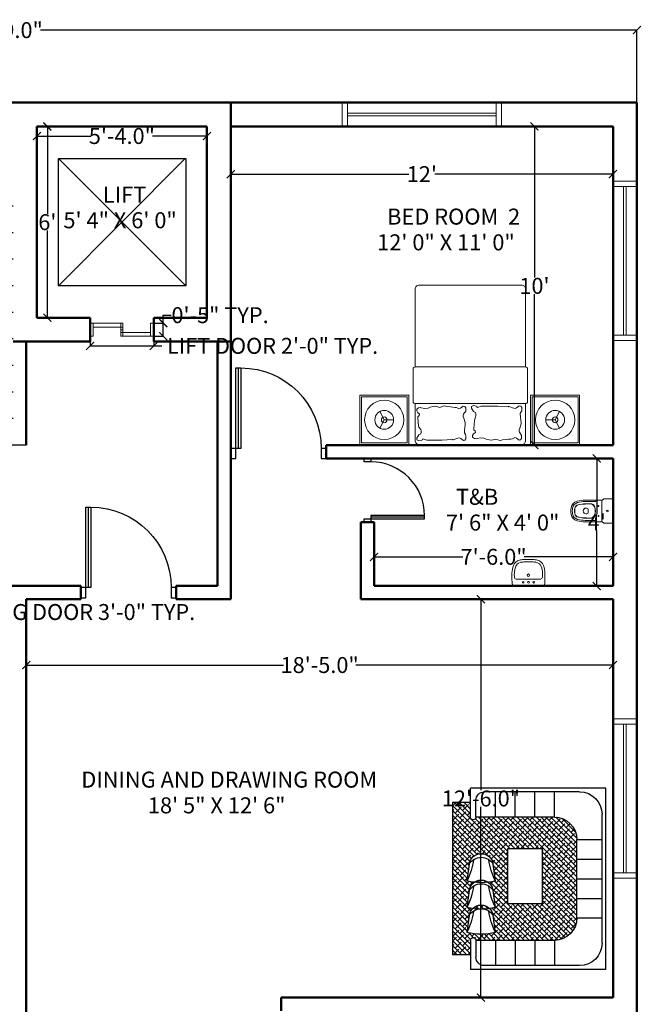
# Model space of a CAD drawing. Units: inches. Extents: x 147 to 1638, y 107 to 941.
# Tile 11 of 17: x 469 to 704, y 570 to 941. Entities that reach past the tile are written whole.
import ezdxf

# ---------------------------------------------------------------- set-up
doc = ezdxf.new("R2010")
doc.units = ezdxf.units.IN
doc.header["$MEASUREMENT"] = 0
for name, color, linetype, lineweight in [('A-ANNO-DIMS', 2, 'Continuous', 15), ('A-AREA-IDEN', 7, 'Continuous', 18), ('A-Door', 150, 'Continuous', 25), ('A-EQPM-ELEV', 7, 'Continuous', 25), ('A-FLOR-FIXT', 9, 'Continuous', 18), ('A-FLOR-STRS', 7, 'Continuous', 25), ('furniture', 50, 'Continuous', 18), ('HAT', 9, 'Continuous', 0), ('lift door', 200, 'Continuous', 20), ('walls', 7, 'Continuous', 50), ('windows', 3, 'Continuous', 20)]:
    doc.layers.add(name, color=color, linetype=linetype, lineweight=lineweight)
for name, color, linetype in [('A-Glaz', 92, 'Continuous'), ('FUR', 42, 'Continuous'), ('NT', 1, 'Continuous'), ('Win', 152, 'Continuous')]:
    doc.layers.add(name, color=color, linetype=linetype)
doc.styles.get("Standard").update_dxf_attribs({"font": 'arial.ttf'})
doc.dimstyles.get("Standard").update_dxf_attribs({"dimtxt": 6, "dimasz": 3, "dimexe": 0.18, "dimexo": 0.0625, "dimgap": 0.09, "dimtad": 0, "dimtih": 1, "dimtoh": 1, "dimdec": 1, "dimzin": 0, "dimdsep": 46, "dimlunit": 3, "dimtxsty": 'Standard', "dimblk": 'ARCHTICK', "dimcen": 0.09, "dimadec": 0, "dimazin": 0, "dimtfac": 1, "dimtdec": 1, "dimtofl": 0, "dimtmove": 0, "dimatfit": 3, "dimfxl": 1, "dimtolj": 1, "dimtzin": 0, "dimarcsym": 0})

# ---------------------------------------------------------------- blocks, each defined once
blk = doc.blocks.new('A$C087A3AA9')
at = {"layer": 'A-Door'}
for points in [[(852.6, 94.7), (852.6, 852.6), (805.3, 852.6), (805.3, 94.7)], [(47.4, 94.7), (47.4, 0), (0, 0), (0, 94.7)], [(900, 94.7), (900, 0), (852.6, 0), (852.6, 94.7)]]:
    blk.add_lwpolyline(points, close=True, dxfattribs=at)
at = {"layer": 'A-Glaz'}
blk.add_line((828.9, 852.6), (828.9, 94.7), dxfattribs=at)
at = {"layer": 'NT'}
blk.add_arc((805.3, 94.7), 757.9, 90, 180, dxfattribs=at)
blk = doc.blocks.new('_ArchTick')
at = {"color": 0, "linetype": 'ByBlock', "const_width": 0.15}
blk.add_lwpolyline([(-0.5, -0.5), (0.5, 0.5)], dxfattribs=at)
blk = doc.blocks.new('*D5')
at = {"layer": 'A-ANNO-DIMS', "color": 0, "lineweight": -2, "transparency": 16777216}
for p, q in [((666.77, 900.72), (663.17, 900.72)), ((663.35, 900.72), (663.35, 843.87)), ((663.35, 780.72), (663.35, 837.56)), ((666.77, 780.72), (663.17, 780.72))]:
    blk.add_line(p, q, dxfattribs=at)
at = {"layer": 'Defpoints', "color": 0, "lineweight": -2, "transparency": 16777216}
for p in [(666.83, 900.72), (663.35, 780.72), (666.83, 780.72)]:
    blk.add_point(p, dxfattribs=at)
at = {"layer": 'A-ANNO-DIMS', "color": 0, "lineweight": -2, "transparency": 16777216, "xscale": 3, "yscale": 3, "zscale": 3}
for p, rotation in [((663.35, 900.72), 90), ((663.35, 780.72), 270)]:
    blk.add_blockref('_ArchTick', p, dxfattribs=dict(at, rotation=rotation))
at = {"layer": 'A-ANNO-DIMS', "color": 0, "transparency": 16777216, "insert": (663.35, 840.72), "char_height": 6, "attachment_point": 5}
blk.add_mtext("\\A1;10'", dxfattribs=at)
blk = doc.blocks.new('*D6')
at = {"layer": 'A-ANNO-DIMS', "color": 0, "lineweight": -2, "transparency": 16777216}
for p, q in [((548.94, 882.79), (616.05, 882.79)), ((548.94, 882.73), (548.94, 882.61)), ((692.94, 882.79), (625.84, 882.79)), ((692.94, 882.85), (692.94, 882.97))]:
    blk.add_line(p, q, dxfattribs=at)
at = {"layer": 'Defpoints', "color": 0, "lineweight": -2, "transparency": 16777216}
for p in [(548.94, 882.79), (692.94, 882.79), (692.94, 882.79)]:
    blk.add_point(p, dxfattribs=at)
at = {"layer": 'A-ANNO-DIMS', "color": 0, "lineweight": -2, "transparency": 16777216, "xscale": 3, "yscale": 3, "zscale": 3, "rotation": 180}
blk.add_blockref('_ArchTick', (548.94, 882.79), dxfattribs=at)
at = {"layer": 'A-ANNO-DIMS', "color": 0, "lineweight": -2, "transparency": 16777216, "xscale": 3, "yscale": 3, "zscale": 3}
blk.add_blockref('_ArchTick', (692.94, 882.79), dxfattribs=at)
at = {"layer": 'A-ANNO-DIMS', "color": 0, "transparency": 16777216, "insert": (620.94, 882.79), "char_height": 6, "attachment_point": 5}
blk.add_mtext("\\A1;12'", dxfattribs=at)
blk = doc.blocks.new('*D10')
at = {"layer": 'A-ANNO-DIMS', "color": 0, "lineweight": -2, "transparency": 16777216}
for p, q in [((687.62, 775.72), (686.65, 775.72)), ((686.83, 775.72), (686.83, 754.81)), ((686.83, 727.72), (686.83, 748.63)), ((687.62, 727.72), (686.65, 727.72))]:
    blk.add_line(p, q, dxfattribs=at)
at = {"layer": 'Defpoints', "color": 0, "lineweight": -2, "transparency": 16777216}
for p in [(687.68, 775.72), (686.83, 727.72), (687.68, 727.72)]:
    blk.add_point(p, dxfattribs=at)
at = {"layer": 'A-ANNO-DIMS', "color": 0, "lineweight": -2, "transparency": 16777216, "xscale": 3, "yscale": 3, "zscale": 3}
for p, rotation in [((686.83, 775.72), 90), ((686.83, 727.72), 270)]:
    blk.add_blockref('_ArchTick', p, dxfattribs=dict(at, rotation=rotation))
at = {"layer": 'A-ANNO-DIMS', "color": 0, "transparency": 16777216, "insert": (686.83, 751.72), "char_height": 6, "attachment_point": 5}
blk.add_mtext("\\A1;4'", dxfattribs=at)
blk = doc.blocks.new('*D11')
at = {"layer": 'A-ANNO-DIMS', "color": 0, "lineweight": -2, "transparency": 16777216}
for p, q in [((602.94, 736.98), (602.94, 738.87)), ((602.94, 738.69), (636.41, 738.69)), ((692.94, 738.69), (659.48, 738.69)), ((692.94, 736.98), (692.94, 738.87))]:
    blk.add_line(p, q, dxfattribs=at)
at = {"layer": 'Defpoints', "color": 0, "lineweight": -2, "transparency": 16777216}
for p in [(692.94, 738.69), (602.94, 736.92), (692.94, 736.92)]:
    blk.add_point(p, dxfattribs=at)
at = {"layer": 'A-ANNO-DIMS', "color": 0, "lineweight": -2, "transparency": 16777216, "xscale": 3, "yscale": 3, "zscale": 3, "rotation": 180}
blk.add_blockref('_ArchTick', (602.94, 738.69), dxfattribs=at)
at = {"layer": 'A-ANNO-DIMS', "color": 0, "lineweight": -2, "transparency": 16777216, "xscale": 3, "yscale": 3, "zscale": 3}
blk.add_blockref('_ArchTick', (692.94, 738.69), dxfattribs=at)
at = {"layer": 'A-ANNO-DIMS', "color": 0, "transparency": 16777216, "insert": (647.94, 738.69), "char_height": 6, "attachment_point": 5}
blk.add_mtext('\\A1;7\'-6.0"', dxfattribs=at)
blk = doc.blocks.new('*D26')
at = {"layer": 'A-ANNO-DIMS', "color": 0, "lineweight": -2, "transparency": 16777216}
for p, q in [((650.57, 722.72), (643.01, 722.72)), ((643.19, 722.72), (643.19, 650.87)), ((643.19, 572.72), (643.19, 644.56)), ((650.57, 572.72), (643.01, 572.72))]:
    blk.add_line(p, q, dxfattribs=at)
at = {"layer": 'Defpoints', "color": 0, "lineweight": -2, "transparency": 16777216}
for p in [(650.64, 722.72), (643.19, 572.72), (650.64, 572.72)]:
    blk.add_point(p, dxfattribs=at)
at = {"layer": 'A-ANNO-DIMS', "color": 0, "lineweight": -2, "transparency": 16777216, "xscale": 3, "yscale": 3, "zscale": 3}
for p, rotation in [((643.19, 722.72), 90), ((643.19, 572.72), 270)]:
    blk.add_blockref('_ArchTick', p, dxfattribs=dict(at, rotation=rotation))
at = {"layer": 'A-ANNO-DIMS', "color": 0, "transparency": 16777216, "insert": (643.19, 647.72), "char_height": 6, "attachment_point": 5}
blk.add_mtext('\\A1;12\'-6.0"', dxfattribs=at)
blk = doc.blocks.new('*D27')
at = {"layer": 'A-ANNO-DIMS', "color": 0, "lineweight": -2, "transparency": 16777216}
for p, q in [((471.94, 695.66), (471.94, 698.14)), ((471.94, 697.96), (568.84, 697.96)), ((692.94, 697.96), (596.05, 697.96)), ((692.94, 695.66), (692.94, 698.14))]:
    blk.add_line(p, q, dxfattribs=at)
at = {"layer": 'Defpoints', "color": 0, "lineweight": -2, "transparency": 16777216}
for p in [(692.94, 697.96), (471.94, 695.6), (692.94, 695.6)]:
    blk.add_point(p, dxfattribs=at)
at = {"layer": 'A-ANNO-DIMS', "color": 0, "lineweight": -2, "transparency": 16777216, "xscale": 3, "yscale": 3, "zscale": 3, "rotation": 180}
blk.add_blockref('_ArchTick', (471.94, 697.96), dxfattribs=at)
at = {"layer": 'A-ANNO-DIMS', "color": 0, "lineweight": -2, "transparency": 16777216, "xscale": 3, "yscale": 3, "zscale": 3}
blk.add_blockref('_ArchTick', (692.94, 697.96), dxfattribs=at)
at = {"layer": 'A-ANNO-DIMS', "color": 0, "transparency": 16777216, "insert": (582.44, 697.96), "char_height": 6, "attachment_point": 5}
blk.add_mtext('\\A1;18\'-5.0"', dxfattribs=at)
blk = doc.blocks.new('*D32')
at = {"layer": 'A-ANNO-DIMS', "color": 0, "lineweight": -2, "transparency": 16777216}
for p, q in [((475.94, 897.2), (475.94, 897.32)), ((539.94, 897.2), (539.94, 897.32)), ((475.94, 897.14), (496.38, 897.14)), ((539.94, 897.14), (519.5, 897.14))]:
    blk.add_line(p, q, dxfattribs=at)
at = {"layer": 'Defpoints', "color": 0, "lineweight": -2, "transparency": 16777216}
for p in [(475.94, 897.14), (539.94, 897.14), (539.94, 897.14)]:
    blk.add_point(p, dxfattribs=at)
at = {"layer": 'A-ANNO-DIMS', "color": 0, "lineweight": -2, "transparency": 16777216, "xscale": 3, "yscale": 3, "zscale": 3, "rotation": 180}
blk.add_blockref('_ArchTick', (475.94, 897.14), dxfattribs=at)
at = {"layer": 'A-ANNO-DIMS', "color": 0, "lineweight": -2, "transparency": 16777216, "xscale": 3, "yscale": 3, "zscale": 3}
blk.add_blockref('_ArchTick', (539.94, 897.14), dxfattribs=at)
at = {"layer": 'A-ANNO-DIMS', "color": 0, "transparency": 16777216, "insert": (507.94, 897.14), "char_height": 6, "attachment_point": 5}
blk.add_mtext('\\A1;5\'-4.0"', dxfattribs=at)
blk = doc.blocks.new('*D33')
at = {"layer": 'A-ANNO-DIMS', "color": 0, "lineweight": -2, "transparency": 16777216}
for p, q in [((479.9, 900.72), (479.68, 900.72)), ((479.86, 900.72), (479.86, 867.87)), ((479.86, 828.72), (479.86, 861.56)), ((479.9, 828.72), (479.68, 828.72))]:
    blk.add_line(p, q, dxfattribs=at)
at = {"layer": 'Defpoints', "color": 0, "lineweight": -2, "transparency": 16777216}
for p in [(479.96, 900.72), (479.86, 828.72), (479.96, 828.72)]:
    blk.add_point(p, dxfattribs=at)
at = {"layer": 'A-ANNO-DIMS', "color": 0, "lineweight": -2, "transparency": 16777216, "xscale": 3, "yscale": 3, "zscale": 3}
for p, rotation in [((479.86, 900.72), 90), ((479.86, 828.72), 270)]:
    blk.add_blockref('_ArchTick', p, dxfattribs=dict(at, rotation=rotation))
at = {"layer": 'A-ANNO-DIMS', "color": 0, "transparency": 16777216, "insert": (479.86, 864.72), "char_height": 6, "attachment_point": 5}
blk.add_mtext("\\A1;6'", dxfattribs=at)
blk = doc.blocks.new('*D69')
at = {"layer": 'A-ANNO-DIMS', "color": 0, "lineweight": -2, "transparency": 16777216}
for p, q in [((224.94, 909.78), (224.94, 937.18)), ((224.94, 937), (449.56, 937)), ((701.94, 937), (477.33, 937)), ((701.94, 909.78), (701.94, 937.18))]:
    blk.add_line(p, q, dxfattribs=at)
at = {"layer": 'Defpoints', "color": 0, "lineweight": -2, "transparency": 16777216}
for p in [(701.94, 937), (224.94, 909.72), (701.94, 909.72)]:
    blk.add_point(p, dxfattribs=at)
at = {"layer": 'A-ANNO-DIMS', "color": 0, "lineweight": -2, "transparency": 16777216, "xscale": 3, "yscale": 3, "zscale": 3, "rotation": 180}
blk.add_blockref('_ArchTick', (224.94, 937), dxfattribs=at)
at = {"layer": 'A-ANNO-DIMS', "color": 0, "lineweight": -2, "transparency": 16777216, "xscale": 3, "yscale": 3, "zscale": 3}
blk.add_blockref('_ArchTick', (701.94, 937), dxfattribs=at)
at = {"layer": 'A-ANNO-DIMS', "color": 0, "transparency": 16777216, "insert": (463.44, 937), "char_height": 6, "attachment_point": 5}
blk.add_mtext('\\A1;39\'-9.0"', dxfattribs=at)
blk = doc.blocks.new('MAT-P14')
for p, q in [((-1.337, 1.348), (-1.337, 1.948)), ((-1.337, 1.948), (-0.737, 1.948)), ((-1.317, 1.928), (-0.757, 1.928)), ((-1.317, 1.368), (-1.317, 1.928)), ((-0.757, 1.368), (-0.757, 1.928)), ((-0.737, 1.348), (-0.737, 1.948)), ((0.625, 1.95), (-0.625, 1.95)), ((0.753, 1.348), (0.753, 1.948)), ((1.353, 1.948), (0.753, 1.948)), ((1.333, 1.928), (0.773, 1.928)), ((0.773, 1.368), (0.773, 1.928)), ((1.333, 1.368), (1.333, 1.928)), ((1.353, 1.348), (1.353, 1.948)), ((-1.037, 1.648), (-1.091, 1.749)), ((1.053, 1.648), (1.108, 1.749)), ((-1.037, 1.648), (-1.091, 1.547)), ((-1.037, 1.648), (-0.922, 1.648)), ((1.053, 1.648), (0.938, 1.648)), ((1.053, 1.648), (1.108, 1.547)), ((-1.337, 1.348), (-0.737, 1.348)), ((-1.317, 1.368), (-0.757, 1.368)), ((1.353, 1.348), (0.753, 1.348)), ((1.333, 1.368), (0.773, 1.368))]:
    blk.add_line(p, q)
for points in [[(-0.675, 1.45), (-0.675, 1.9, -0.414214), (-0.625, 1.95), (0.625, 1.95, -0.414214), (0.675, 1.9), (0.675, 1.45)], [(-0.675, 1, -0.414214), (-0.7, 1.025), (-0.7, 1.425, -0.414214), (-0.675, 1.45), (0.675, 1.45, -0.414214), (0.7, 1.425), (0.7, 1.025, -0.414214), (0.675, 1)], [(-0.625, 0, -0.414214), (-0.675, 0.05), (-0.675, 1), (0.675, 1), (0.675, 0.05, -0.414214), (0.625, 0)]]:
    blk.add_lwpolyline(points, format="xyb", close=True)
blk.add_lwpolyline([(-0.542, 1.95), (-0.542, 1.967), (0.558, 1.967), (0.558, 1.95)], close=True)
for points in [[(-0.614, 1.818), (-0.626, 1.838), (-0.626, 1.877), (-0.614, 1.891), (-0.596, 1.896), (-0.579, 1.886), (-0.563, 1.872), (-0.545, 1.863), (-0.516, 1.879), (-0.497, 1.882), (-0.465, 1.884), (-0.439, 1.887), (-0.395, 1.892), (-0.363, 1.9), (-0.309, 1.882), (-0.262, 1.897), (-0.23, 1.892), (-0.192, 1.884), (-0.166, 1.873), (-0.128, 1.868), (-0.082, 1.875), (-0.076, 1.88), (-0.052, 1.875), (-0.028, 1.861), (-0.028, 1.841), (-0.04, 1.817), (-0.064, 1.802), (-0.06, 1.781), (-0.043, 1.768), (-0.046, 1.697), (-0.05, 1.662), (-0.056, 1.64), (-0.062, 1.612), (-0.068, 1.596), (-0.068, 1.579), (-0.063, 1.56), (-0.039, 1.545), (-0.015, 1.505), (-0.015, 1.486), (-0.038, 1.471), (-0.075, 1.482), (-0.081, 1.487), (-0.087, 1.497), (-0.134, 1.481), (-0.304, 1.482), (-0.318, 1.482), (-0.335, 1.479), (-0.464, 1.488), (-0.467, 1.486), (-0.473, 1.486), (-0.517, 1.503), (-0.53, 1.505), (-0.548, 1.51), (-0.566, 1.501), (-0.581, 1.487), (-0.599, 1.477), (-0.617, 1.482), (-0.629, 1.497), (-0.629, 1.536), (-0.623, 1.55), (-0.611, 1.57), (-0.614, 1.614), (-0.615, 1.627), (-0.618, 1.644), (-0.619, 1.66), (-0.62, 1.675), (-0.62, 1.695), (-0.618, 1.707), (-0.614, 1.723), (-0.608, 1.739), (-0.604, 1.75), (-0.598, 1.771), (-0.596, 1.785), (-0.6, 1.798), (-0.614, 1.819)], [(0.069, 1.559), (0.057, 1.54), (0.057, 1.501), (0.069, 1.486), (0.087, 1.481), (0.105, 1.491), (0.121, 1.505), (0.139, 1.514), (0.168, 1.498), (0.187, 1.496), (0.219, 1.493), (0.244, 1.49), (0.289, 1.485), (0.321, 1.477), (0.374, 1.495), (0.422, 1.48), (0.454, 1.486), (0.492, 1.493), (0.517, 1.504), (0.555, 1.509), (0.602, 1.502), (0.608, 1.497), (0.632, 1.502), (0.656, 1.517), (0.656, 1.536), (0.644, 1.561), (0.62, 1.575), (0.624, 1.596), (0.641, 1.609), (0.637, 1.68), (0.633, 1.715), (0.628, 1.738), (0.606, 1.765), (0.6, 1.781), (0.6, 1.798), (0.605, 1.817), (0.629, 1.832), (0.654, 1.872), (0.654, 1.892), (0.63, 1.906), (0.593, 1.895), (0.587, 1.891), (0.581, 1.881), (0.534, 1.896), (0.379, 1.896), (0.366, 1.896), (0.348, 1.898), (0.22, 1.89), (0.216, 1.891), (0.21, 1.891), (0.167, 1.875), (0.154, 1.872), (0.136, 1.867), (0.118, 1.876), (0.102, 1.89), (0.085, 1.9), (0.067, 1.895), (0.055, 1.881), (0.055, 1.842), (0.061, 1.827), (0.073, 1.807), (0.07, 1.764), (0.069, 1.75), (0.066, 1.733), (0.065, 1.718), (0.063, 1.703), (0.063, 1.682), (0.066, 1.67), (0.07, 1.655), (0.075, 1.638), (0.079, 1.627), (0.086, 1.607), (0.087, 1.592), (0.083, 1.579), (0.07, 1.559)]]:
    blk.add_lwpolyline(points)
for centre, radius in [((-1.037, 1.648), 0.24), ((1.053, 1.648), 0.24), ((-1.037, 1.648), 0.115), ((1.053, 1.648), 0.115), ((-1.037, 1.648), 0.035), ((1.053, 1.648), 0.035)]:
    blk.add_circle(centre, radius)
blk = doc.blocks.new('2SAINDA')
at = {"color": 0, "linetype": 'ByBlock'}
for p, q in [((0, 0.188), (0, -0.188)), ((0.018, 0.2), (0.141, 0.2)), ((0.157, 0.192), (0.162, 0.188)), ((0.18, -0.164), (0.18, 0.164)), ((0.279, 0.159), (0.261, 0.176)), ((0.437, 0.047), (0.424, 0.047)), ((0.279, -0.159), (0.261, -0.176)), ((0.437, -0.047), (0.424, -0.047)), ((0.018, -0.2), (0.141, -0.2)), ((0.157, -0.192), (0.162, -0.188))]:
    blk.add_line(p, q, dxfattribs=at)
for centre, radius in [((0.09, 0), 0.0135), ((0.09, 0), 0.0135), ((0.236, 0.08), 0.0075), ((0.236, -0.08), 0.0075)]:
    blk.add_circle(centre, radius, dxfattribs=at)
for centre, radius, start, end in [((0.018, 0.18), 0.02, 90, 155.6901), ((0.141, 0.181), 0.019, 34.9372, 90), ((0.155, 0.164), 0.025, 23.3776, 73.7848), ((0.383, -5.322), 5.5, 89.2905, 92.1362), ((0.155, 0.164), 0.025, 360, 23.3776), ((0.444, -0.373), 0.55, 75.4605, 89.2905), ((0.293, 0.173), 0.02, 225, 270.9364), ((0.485, 0), 0.2, 160.016, 199.984), ((0.485, 0), 0.196, 160.016, 199.984), ((0.383, -5.322), 5.476, 89.2905, 90.9364), ((0.368, 0.043), 0.075, 90.1648, 160.016), ((0.368, 0.043), 0.071, 90.1648, 160.016), ((0.383, -5.322), 5.44, 89.2905, 90.1648), ((0.383, -5.322), 5.436, 89.2905, 90.1648), ((0.582, 0), 0.18, 170.2849, 189.7151), ((0.424, 0.027), 0.02, 90, 170.2849), ((0.437, 0), 0.047, 0, 90), ((0.437, 0), 0.047, 270, 0), ((0.444, -0.373), 0.49, 75.4605, 89.2905), ((0.444, -0.373), 0.486, 75.4605, 89.2905), ((0.444, -0.373), 0.526, 75.4605, 89.2905), ((0.549, 0.03), 0.07, 8.8162, 75.4605), ((0.549, 0.03), 0.074, 8.8162, 75.4605), ((0.549, 0.03), 0.11, 8.8162, 75.4605), ((0.549, 0.03), 0.134, 8.8162, 75.4605), ((0.355, 0), 0.266, 351.1838, 8.8162), ((0.355, 0), 0.27, 351.1838, 8.8162), ((0.355, 0), 0.306, 351.1838, 8.8162), ((0.355, 0), 0.33, 351.1838, 8.8162), ((0.293, -0.173), 0.02, 89.0636, 135), ((0.383, 5.322), 5.476, 269.0636, 270.7095), ((0.368, -0.043), 0.075, 199.984, 269.8352), ((0.368, -0.043), 0.071, 199.984, 269.8352), ((0.383, 5.322), 5.436, 269.8352, 270.7095), ((0.383, 5.322), 5.44, 269.8352, 270.7095), ((0.424, -0.027), 0.02, 189.7151, 270), ((0.444, 0.373), 0.486, 270.7095, 284.5395), ((0.444, 0.373), 0.49, 270.7095, 284.5395), ((0.444, 0.373), 0.526, 270.7095, 284.5395), ((0.444, 0.373), 0.55, 270.7095, 284.5395), ((0.549, -0.03), 0.07, 284.5395, 351.1838), ((0.549, -0.03), 0.074, 284.5395, 351.1838), ((0.549, -0.03), 0.11, 284.5395, 351.1838), ((0.549, -0.03), 0.134, 284.5395, 351.1838), ((0.018, -0.18), 0.02, 204.3099, 270), ((0.141, -0.181), 0.019, 270, 325.0628), ((0.155, -0.164), 0.025, 286.2152, 336.6224), ((0.155, -0.164), 0.025, 336.6224, 0), ((0.383, 5.322), 5.5, 267.8638, 270.7095)]:
    blk.add_arc(centre, radius, start, end, dxfattribs=at)
blk = doc.blocks.new('2SALADA2')
at = {"color": 0}
for p, q in [((-0.296, 0), (0.296, 0)), ((0.207, -0.13), (-0.207, -0.13))]:
    blk.add_line(p, q, dxfattribs=at)
for centre, radius in [((-0.1, -0.07), 0.015), ((0, -0.205), 0.023), ((0, -0.07), 0.0175), ((0.1, -0.07), 0.015)]:
    blk.add_circle(centre, radius, dxfattribs=at)
for centre, radius, start, end in [((-0.296, -0.01), 0.01, 90, 173.6262), ((0.296, -0.01), 0.01, 6.3738, 90), ((1.185, -0.175), 1.5, 173.6262, 182.693), ((1.186, -0.221), 1.454, 178.0234, 180.898), ((-0.227, -0.171), 0.04, 95.5937, 179.6995), ((-0.207, -0.38), 0.25, 90, 95.5937), ((0.207, -0.38), 0.25, 84.4063, 90), ((0.227, -0.171), 0.04, 0.3005, 84.4063), ((-1.186, -0.221), 1.454, 359.102, 1.9766), ((-1.185, -0.175), 1.5, 357.307, 6.3738), ((0.186, -0.222), 0.5, 182.693, 199.3406), ((0.186, -0.222), 0.454, 182.693, 199.3406), ((-0.135, -0.335), 0.114, 199.3406, 257.4429), ((0.135, -0.335), 0.114, 282.5571, 340.6594), ((-0.186, -0.222), 0.454, 340.6594, 357.307), ((-0.186, -0.222), 0.5, 340.6594, 357.307), ((-0.135, -0.335), 0.16, 199.3406, 257.4429), ((-0.061, -0.003), 0.5, 257.4429, 266.4982), ((-0.061, -0.003), 0.454, 257.4429, 266.4982), ((0, 0.995), 1.5, 266.4982, 273.5018), ((0, 0.995), 1.454, 266.4982, 273.5018), ((0.061, -0.003), 0.454, 273.5018, 282.5571), ((0.061, -0.003), 0.5, 273.5018, 282.5571), ((0.135, -0.335), 0.16, 282.5571, 340.6594)]:
    blk.add_arc(centre, radius, start, end, dxfattribs=at)
blk = doc.blocks.new('CHAIR1')
for p, q in [((-393, -750), (-329, -287)), ((329, -286), (394, -750))]:
    blk.add_line(p, q)
for centre, radius, start, end in [((0, -332), 332, 7.9072, 172.1612), ((-1856, 27), 1657, 332.0394, 353.4161), ((0, -483), 383, 30.9021, 149.1663), ((1857, 27), 1657, 186.5839, 207.9606), ((0, 770), 1570, 255.502, 284.498)]:
    blk.add_arc(centre, radius, start, end)
blk = doc.blocks.new('A$C1CFC4E3A')
at = {"layer": 'HAT'}
h = blk.add_hatch(dxfattribs=at)
h.set_pattern_fill('ANSI38,_O', color=256, scale=0.664121)
h.set_pattern_definition([(45, (6.13299, -18.48134), (-0.05870057, 0.05870057), []), (135, (6.13299, -18.48134), (-0.1761017, 0.05870057), [0.2075378, -0.1245227])])
h.paths.add_polyline_path([(0, 3.705), (-0.438, 3.705), (-0.438, 3.353, -1), (-0.573, 3.353), (-2.482, 3.353, 0.414214), (-3.028, 2.807), (-3.028, 0.898, 0.414214), (-2.482, 0.352), (-0.573, 0.352, -1), (-0.438, 0.352), (-0.438, 0), (0, 0)])
h.paths.add_polyline_path([(-1.342, 1.248), (-2.191, 1.248), (-2.191, 2.58), (-1.342, 2.58)], flags=16)
h.paths.add_polyline_path([(-0.409, 1.566), (-0.352, 1.156, -0.127199), (-1.048, 1.156), (-0.992, 1.566, -0.871235)], flags=16)
h.paths.add_polyline_path([(-0.409, 0.959), (-0.352, 0.548, -0.127199), (-1.048, 0.548), (-0.992, 0.958, -0.871235)], flags=16)
h.paths.add_polyline_path([(-0.992, 2.209, -0.871235), (-0.409, 2.21), (-0.352, 1.799, -0.127199), (-1.048, 1.799)], flags=16)
at = {"layer": 'FUR'}
for p, q in [((-3.732, 4.057), (-0.438, 4.057)), ((-3.732, -0.352), (-3.732, 4.057)), ((-3.096, 3.967), (-0.777, 3.967)), ((-2.482, 3.353), (-2.482, 3.967)), ((-2.005, 3.353), (-2.005, 3.967)), ((-1.528, 3.353), (-1.528, 3.967)), ((-1.05, 3.353), (-1.05, 3.967)), ((-0.438, 3.353), (-0.438, 4.057)), ((-0.573, 3.353), (-0.573, 3.762)), ((-3.642, 0.284), (-3.642, 3.421)), ((-2.482, 3.353), (-0.573, 3.353)), ((-3.028, 2.807), (-3.642, 2.807)), ((-3.028, 2.33), (-3.642, 2.33)), ((-3.028, 1.852), (-3.642, 1.852)), ((-3.028, 1.375), (-3.642, 1.375)), ((-3.028, 0.898), (-3.642, 0.898)), ((-2.482, 0.352), (-0.573, 0.352)), ((-2.482, 0.352), (-2.482, -0.262)), ((-2.005, 0.352), (-2.005, -0.262)), ((-1.528, 0.352), (-1.528, -0.262)), ((-1.05, 0.352), (-1.05, -0.262)), ((-0.573, 0.352), (-0.573, -0.057)), ((-0.438, 0.352), (-0.438, -0.352)), ((-3.732, -0.352), (-0.438, -0.352)), ((-3.096, -0.262), (-0.777, -0.262))]:
    blk.add_line(p, q, dxfattribs=at)
for centre, radius, start, end in [((-3.096, 3.421), 0.546, 90, 180), ((-0.777, 3.762), 0.205, 0, 90), ((-2.482, 2.807), 0.546, 90, 180), ((-0.505, 3.353), 0.0675, 180, 0), ((-2.482, 0.898), 0.546, 180, 270), ((-3.096, 0.284), 0.546, 180, 270), ((-0.505, 0.352), 0.0675, 0, 180), ((-0.777, -0.057), 0.205, 270, 0)]:
    blk.add_arc(centre, radius, start, end, dxfattribs=at)
at = {"layer": 'Win'}
for p, q in [((-0.438, 3.705), (0, 3.705)), ((0, 3.705), (0, 0)), ((-3.028, 0.898), (-3.028, 2.807)), ((-0.438, 0), (0, 0))]:
    blk.add_line(p, q, dxfattribs=at)
blk.add_lwpolyline([(-2.191, 2.58), (-1.342, 2.58), (-1.342, 1.248), (-2.191, 1.248)], close=True, dxfattribs=at)
at = {"layer": 'FUR', "xscale": 0.0008854948152227, "yscale": 0.0008854948152227, "zscale": 0.0008854948152227}
for p in [(-0.7, 2.463), (-0.7, 1.82), (-0.7, 1.212)]:
    blk.add_blockref('CHAIR1', p, dxfattribs=at)
blk = doc.blocks.new('WIN-60IN')
for p, q in [((60, 9), (0, 9)), ((0, 9), (0, 0)), ((2, 9), (2, 0)), ((58, 0), (58, 9)), ((60, 0), (60, 9)), ((2, 5), (58, 5)), ((2, 4), (58, 4)), ((0, 0), (60, 0))]:
    blk.add_line(p, q)
blk = doc.blocks.new('LIFT-CAR')
for p, q in [((48, 0), (0, 48)), ((47.77, 48), (0, 0))]:
    blk.add_line(p, q)
blk.add_lwpolyline([(0, 48), (48, 48), (48, 0), (0, 0)], close=True)
blk = doc.blocks.new('LIFT-DOOR-CENTER-OPEN')
for p, q in [((1.24, 4.95), (12.38, 4.95)), ((11.62, 2.48), (11.62, 4.95)), ((12.38, 4.95), (12.38, 2.48)), ((1.24, 3.49), (12.38, 3.49)), ((11.62, 0), (11.62, 2.48)), ((11.62, 2.48), (12.38, 2.48)), ((12.38, 2.48), (11.62, 2.48)), ((22.76, 1.47), (11.62, 1.47)), ((12.38, 2.48), (12.38, 0)), ((22.76, 0), (11.62, 0))]:
    blk.add_line(p, q)
for points in [[(1.24, 0), (0, 0), (0, 4.95), (1.24, 4.95)], [(22.76, 4.95), (24, 4.95), (24, 0), (22.76, 0)]]:
    blk.add_lwpolyline(points, close=True)
blk = doc.blocks.new('STAIR-RETURN-FLIGHTS')
for p, q in [((0, 90), (36, 90)), ((36, 0), (36, 90)), ((36, 90), (48, 90)), ((84, 90), (48, 90)), ((48, 90), (48, 0)), ((0, 80), (36, 80)), ((84, 80), (48, 80)), ((0, 70), (36, 70)), ((84, 70), (48, 70)), ((0, 60), (36, 60)), ((84, 60), (48, 60)), ((0, 50), (36, 50)), ((84, 50), (48, 50)), ((0, 40), (36, 40)), ((84, 40), (48, 40)), ((0, 30), (36, 30)), ((84, 30), (48, 30)), ((0, 20), (36, 20)), ((84, 20), (48, 20)), ((0, 10), (36, 10)), ((84, 10), (48, 10)), ((0, 0), (36, 0)), ((48, 0), (36, 0)), ((89, 0), (48, 0))]:
    blk.add_line(p, q)
blk = doc.blocks.new('*D100')
at = {"layer": 'A-ANNO-DIMS', "color": 0, "lineweight": -2, "transparency": 16777216}
for p, q in [((404.44, 723.26), (404.44, 717.74)), ((440.44, 723.26), (440.44, 717.74)), ((404.44, 717.92), (440.44, 717.92)), ((440.44, 717.92), (443.44, 717.92))]:
    blk.add_line(p, q, dxfattribs=at)
at = {"layer": 'Defpoints', "color": 0, "lineweight": -2, "transparency": 16777216}
for p in [(404.44, 723.32), (440.44, 723.32), (440.44, 717.92)]:
    blk.add_point(p, dxfattribs=at)
at = {"layer": 'A-ANNO-DIMS', "color": 0, "lineweight": -2, "transparency": 16777216, "xscale": 3, "yscale": 3, "zscale": 3, "rotation": 180}
blk.add_blockref('_ArchTick', (404.44, 717.92), dxfattribs=at)
at = {"layer": 'A-ANNO-DIMS', "color": 0, "lineweight": -2, "transparency": 16777216, "xscale": 3, "yscale": 3, "zscale": 3}
blk.add_blockref('_ArchTick', (440.44, 717.92), dxfattribs=at)
at = {"layer": 'A-ANNO-DIMS', "color": 0, "transparency": 16777216, "insert": (490.91, 717.92), "char_height": 6, "attachment_point": 5}
blk.add_mtext('\\A1;SWING DOOR 3\'-0" TYP.', dxfattribs=at)
blk = doc.blocks.new('*D130')
at = {"layer": 'A-ANNO-DIMS', "color": 0, "lineweight": -2, "transparency": 16777216}
for p, q in [((495.94, 821.68), (495.94, 817.96)), ((519.94, 821.68), (519.94, 817.96)), ((495.94, 818.14), (519.94, 818.14)), ((519.94, 818.14), (522.94, 818.14))]:
    blk.add_line(p, q, dxfattribs=at)
at = {"layer": 'Defpoints', "color": 0, "lineweight": -2, "transparency": 16777216}
for p in [(495.94, 821.74), (519.94, 821.74), (519.94, 818.14)]:
    blk.add_point(p, dxfattribs=at)
at = {"layer": 'A-ANNO-DIMS', "color": 0, "lineweight": -2, "transparency": 16777216, "xscale": 3, "yscale": 3, "zscale": 3, "rotation": 180}
blk.add_blockref('_ArchTick', (495.94, 818.14), dxfattribs=at)
at = {"layer": 'A-ANNO-DIMS', "color": 0, "lineweight": -2, "transparency": 16777216, "xscale": 3, "yscale": 3, "zscale": 3}
blk.add_blockref('_ArchTick', (519.94, 818.14), dxfattribs=at)
at = {"layer": 'A-ANNO-DIMS', "color": 0, "transparency": 16777216, "insert": (564.7, 818.14), "char_height": 6, "attachment_point": 5}
blk.add_mtext('\\A1;LIFT DOOR 2\'-0" TYP.', dxfattribs=at)
blk = doc.blocks.new('*D131')
at = {"layer": 'A-ANNO-DIMS', "color": 0, "lineweight": -2, "transparency": 16777216}
for p, q in [((523.54, 826.69), (523.54, 829.69)), ((523.54, 829.69), (526.54, 829.69)), ((520.01, 826.69), (523.72, 826.69)), ((523.54, 821.74), (523.54, 826.69)), ((520.01, 821.74), (523.72, 821.74))]:
    blk.add_line(p, q, dxfattribs=at)
at = {"layer": 'Defpoints', "color": 0, "lineweight": -2, "transparency": 16777216}
for p in [(519.94, 826.69), (523.54, 826.69), (519.94, 821.74)]:
    blk.add_point(p, dxfattribs=at)
at = {"layer": 'A-ANNO-DIMS', "color": 0, "lineweight": -2, "transparency": 16777216, "xscale": 3, "yscale": 3, "zscale": 3}
for p, rotation in [((523.54, 826.69), 90), ((523.54, 821.74), 270)]:
    blk.add_blockref('_ArchTick', p, dxfattribs=dict(at, rotation=rotation))
at = {"layer": 'A-ANNO-DIMS', "color": 0, "transparency": 16777216, "insert": (544.92, 829.69), "char_height": 6, "attachment_point": 5}
blk.add_mtext('\\A1;0\'-5" TYP.', dxfattribs=at)

msp = doc.modelspace()

# ---------------------------------------------------------------- linework, layer by layer
at = {"layer": 'walls'}
for p, q in [((224.94, 909.72), (701.94, 909.72)), ((548.94, 909.72), (548.94, 780.72)), ((701.94, 909.72), (701.94, 201.72)), ((475.94, 900.72), (539.94, 900.72)), ((475.94, 900.72), (475.94, 828.72)), ((539.94, 900.72), (539.94, 828.72)), ((548.94, 900.72), (692.94, 900.72)), ((692.94, 900.72), (692.94, 780.72)), ((475.94, 828.72), (495.94, 828.72)), ((495.94, 828.72), (495.94, 819.72)), ((519.94, 828.72), (519.94, 819.72)), ((519.94, 828.72), (539.94, 828.72)), ((466.94, 819.72), (495.94, 819.72)), ((471.94, 819.72), (471.94, 780.72)), ((519.94, 819.72), (548.94, 819.72)), ((543.94, 819.72), (543.94, 727.72)), ((548.94, 775.72), (548.94, 780.72)), ((584.94, 780.72), (692.94, 780.72)), ((584.94, 775.72), (584.94, 780.72)), ((548.94, 775.72), (548.94, 722.72)), ((584.94, 775.72), (597.94, 775.72)), ((597.94, 775.72), (602.94, 775.72)), ((602.94, 775.72), (692.94, 775.72)), ((692.94, 775.72), (692.94, 727.72)), ((597.94, 751.72), (597.94, 722.72)), ((597.94, 751.72), (602.94, 751.72)), ((602.94, 751.72), (602.94, 727.72)), ((440.44, 727.72), (492.44, 727.72)), ((492.44, 722.72), (492.44, 727.72)), ((528.44, 722.72), (528.44, 727.72)), ((528.44, 727.72), (543.94, 727.72)), ((602.94, 727.72), (692.94, 727.72)), ((471.94, 722.72), (471.94, 400.72)), ((471.94, 722.72), (492.44, 722.72)), ((528.44, 722.72), (548.94, 722.72)), ((597.94, 722.72), (692.94, 722.72)), ((692.94, 722.72), (692.94, 572.72)), ((567.94, 572.72), (567.94, 567.72)), ((567.94, 572.72), (692.94, 572.72))]:
    msp.add_line(p, q, dxfattribs=at)

# ---------------------------------------------------------------- block references
at = {"layer": 'A-Door', "xscale": -0.0400000000000001, "yscale": 0.0400000000000001, "zscale": 0.0400000000000001}
for p in [(584.94, 775.72), (528.44, 723.32)]:
    msp.add_blockref('A$C087A3AA9', p, dxfattribs=at)
at = {"layer": 'A-Door', "xscale": 0.0266666667542921, "yscale": 0.0266666667542921, "zscale": 0.0266666667542921, "rotation": 270}
msp.add_blockref('A$C087A3AA9', (599.21, 775.72), dxfattribs=at)
at = {"layer": 'A-EQPM-ELEV'}
msp.add_blockref('LIFT-CAR', (484.06, 840.72), dxfattribs=at)
at = {"layer": 'A-FLOR-FIXT', "rotation": 180}
for name, p, xscale, yscale, zscale in [('2SAINDA', (692.94, 755.96), 23.19012112898009, 23.19012112898009, 23.19012112898009), ('2SALADA2', (661.08, 727.72), 19.81841434140962, 19.81841434140962, 19.81841434140962)]:
    msp.add_blockref(name, p, dxfattribs=dict(at, xscale=xscale, yscale=yscale, zscale=zscale))
at = {"layer": 'A-FLOR-STRS'}
msp.add_blockref('STAIR-RETURN-FLIGHTS', (382.94, 780.72), dxfattribs=at)
at = {"layer": 'furniture', "xscale": 30.80045642108221, "yscale": 30.80045642108221, "zscale": 30.80045642108221, "rotation": 180}
msp.add_blockref('MAT-P14', (639.2, 841.03), dxfattribs=at)
at = {"layer": 'furniture', "xscale": -15.47145176415956, "yscale": 15.47145176415956, "zscale": 15.47145176415956}
msp.add_blockref('A$C1CFC4E3A', (632.46, 588.83), dxfattribs=at)
at = {"layer": 'lift door'}
msp.add_blockref('LIFT-DOOR-CENTER-OPEN', (495.94, 821.74), dxfattribs=at)
at = {"layer": 'windows'}
for p, rotation in [((650.94, 909.72), 180), ((692.94, 880.14), 270.0000000000002), ((692.94, 677.72), 270.0000000000002)]:
    msp.add_blockref('WIN-60IN', p, dxfattribs=dict(at, rotation=rotation))

# ---------------------------------------------------------------- texts
at = {"layer": 'A-AREA-IDEN'}
for s, height, p in [('LIFT', 6.031, (500.77, 872.01)), (' 5\' 4" X 6\' 0"', 6.0306, (484.06, 862.41)), ('BED ROOM  2', 6.0306, (607.85, 863.78)), ('  12\' 0" X 11\' 0"', 6.0306, (600.4, 854.09)), ('T&B', 6.031, (633.78, 758.28)), ('  7\' 6" X 4\' 0"', 6.0306, (626.33, 748.59)), ('DINING AND DRAWING ROOM', 6.0306, (492.65, 651.8)), ('18\' 5" X 12\' 6"', 6.0306, (517.72, 642.11))]:
    msp.add_text(s, height=height, dxfattribs=at).set_placement(p)

# ---------------------------------------------------------------- dimensions: what is measured, and where the dimension line sits
at = {"layer": 'A-ANNO-DIMS'}
for base, p1, p2, picture, middle in [((701.94, 937), (224.94, 909.72), (701.94, 909.72), '*D69', (463.44, 937)), ((539.94, 897.14), (475.94, 897.14), (539.94, 897.14), '*D32', (507.94, 897.14)), ((692.94, 882.79), (548.94, 882.79), (692.94, 882.79), '*D6', (620.94, 882.79)), ((692.94, 738.69), (602.94, 736.92), (692.94, 736.92), '*D11', (647.94, 738.69)), ((692.94, 697.96), (471.94, 695.6), (692.94, 695.6), '*D27', (582.44, 697.96))]:
    dim = msp.add_linear_dim(base=base, p1=p1, p2=p2, dimstyle='Standard', override={"dimclrd": 0, "dimclre": 0, "dimclrt": 0}, dxfattribs=at)
    dim.commit()
    dim.dimension.update_dxf_attribs({"geometry": picture, "text_midpoint": middle})
for base, p1, p2, picture, middle in [((479.86, 828.72), (479.96, 900.72), (479.96, 828.72), '*D33', (479.86, 864.72)), ((663.35, 780.72), (666.83, 900.72), (666.83, 780.72), '*D5', (663.35, 840.72)), ((686.83, 727.72), (687.68, 775.72), (687.68, 727.72), '*D10', (686.83, 751.72)), ((643.19, 572.72), (650.64, 722.72), (650.64, 572.72), '*D26', (643.19, 647.72))]:
    dim = msp.add_linear_dim(base=base, p1=p1, p2=p2, angle=90, dimstyle='Standard', override={"dimclrd": 0, "dimclre": 0, "dimclrt": 0}, dxfattribs=at)
    dim.commit()
    dim.dimension.update_dxf_attribs({"geometry": picture, "text_midpoint": middle})
dim = msp.add_linear_dim(base=(523.544, 826.6944), p1=(519.944, 821.7415), p2=(519.944, 826.6944), angle=90, text='<> TYP.', dimstyle='Standard', override={"dimdec": 1, "dimlfac": 1, "dimrnd": 0, "dimzin": 1, "dimdsep": 46, "dimlunit": 4, "dimfrac": 2}, dxfattribs=at)
dim.commit()
dim.dimension.update_dxf_attribs({"geometry": '*D131', "text_midpoint": (544.9205, 829.6944)})
for base, p1, p2, text, picture, middle in [((519.94, 818.14), (495.94, 821.74), (519.94, 821.74), 'LIFT DOOR <> TYP.', '*D130', (564.7, 818.14)), ((440.44, 717.92), (404.44, 723.32), (440.44, 723.32), 'SWING DOOR <> TYP.', '*D100', (490.91, 717.92))]:
    dim = msp.add_linear_dim(base=base, p1=p1, p2=p2, text=text, dimstyle='Standard', override={"dimdec": 1, "dimlfac": 1, "dimrnd": 0, "dimzin": 1, "dimdsep": 46, "dimlunit": 4, "dimfrac": 2}, dxfattribs=at)
    dim.commit()
    dim.dimension.update_dxf_attribs({"geometry": picture, "text_midpoint": middle})

doc.saveas('drawing.dxf')
